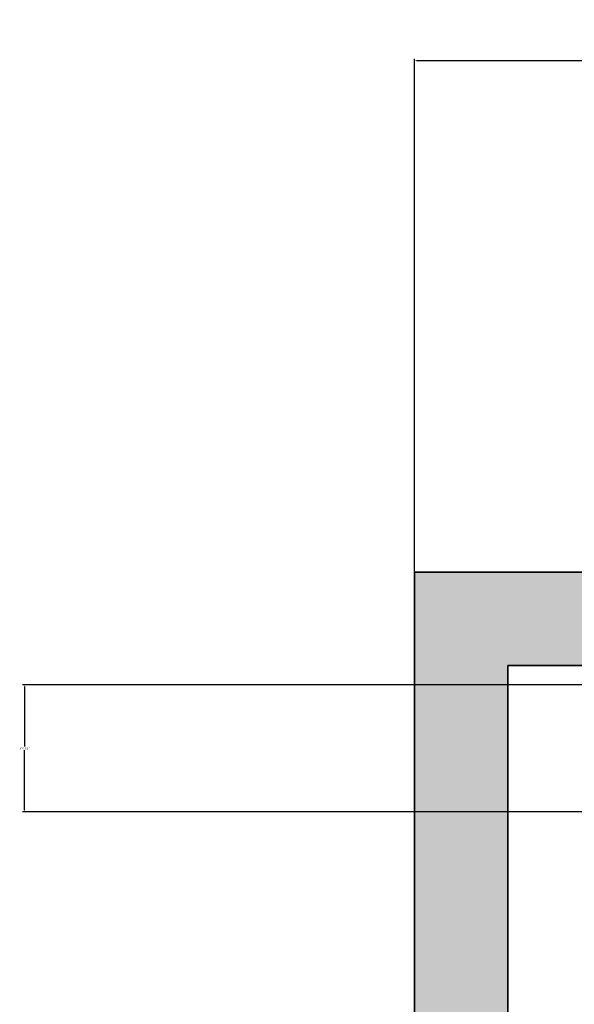
# Model space of a CAD drawing. Units: inches. Extents: x -5 to 482, y -460 to 66.
# Tile 23 of 31: x -5 to 48, y -29 to 66. Entities that reach past the tile are written whole.
import ezdxf

# ---------------------------------------------------------------- set-up
doc = ezdxf.new("R2010")
doc.units = ezdxf.units.IN
doc.header["$MEASUREMENT"] = 0
for name, color, linetype, lineweight in [('A-ANNO-DIMS', 2, 'Continuous', 18), ('A-WALL', 7, 'Continuous', 35), ('A-WALL-PATT', 152, 'Continuous', 13)]:
    doc.layers.add(name, color=color, linetype=linetype, lineweight=lineweight)
doc.styles.get("Standard").update_dxf_attribs({"font": 'arial.ttf'})
doc.dimstyles.get("Standard").update_dxf_attribs({"dimtxt": 0.18, "dimasz": 0.18, "dimexe": 0.18, "dimexo": 0.0625, "dimgap": 0.09, "dimtad": 0, "dimtih": 1, "dimtoh": 1, "dimdec": 0, "dimzin": 0, "dimdsep": 46, "dimlunit": 3, "dimtxsty": 'Standard', "dimcen": 0.09, "dimadec": 0, "dimazin": 0, "dimtfac": 1, "dimtdec": 0, "dimtofl": 0, "dimtmove": 0, "dimatfit": 3, "dimfxl": 1, "dimtolj": 1, "dimtzin": 0, "dimarcsym": 0})

# ---------------------------------------------------------------- blocks, each defined once
blk = doc.blocks.new('*D3')
at = {"layer": 'A-ANNO-DIMS', "color": 0, "lineweight": -2, "transparency": 16777216}
for p, q in [((32.877, 13.214), (32.877, 62.612)), ((33.057, 62.432), (221.233, 62.432)), ((430.197, 62.432), (242.02, 62.432)), ((430.377, 13.214), (430.377, 62.612))]:
    blk.add_line(p, q, dxfattribs=at)
at = {"layer": 'A-ANNO-DIMS', "color": 0, "transparency": 16777216}
for points in [[(33.057, 62.462), (33.057, 62.402), (32.877, 62.432)], [(430.197, 62.462), (430.197, 62.402), (430.377, 62.432)]]:
    blk.add_solid(points, dxfattribs=at)
at = {"layer": 'Defpoints', "color": 0, "transparency": 16777216}
for p in [(430.377, 62.432), (32.877, 13.151), (430.377, 13.151)]:
    blk.add_point(p, dxfattribs=at)
at = {"layer": 'A-ANNO-DIMS', "color": 0, "transparency": 16777216, "insert": (231.627, 62.432), "char_height": 6, "attachment_point": 5}
blk.add_mtext('\\A1;33\'-2"', dxfattribs=at)
blk = doc.blocks.new('*D70')
at = {"layer": 'A-ANNO-DIMS', "color": 0, "lineweight": -2, "transparency": 16777216}
for p, q in [((83.652, 2.288), (-4.903, 2.288)), ((-4.723, 2.108), (-4.723, -3.659)), ((-4.723, -9.792), (-4.723, -4.025)), ((83.652, -9.972), (-4.903, -9.972))]:
    blk.add_line(p, q, dxfattribs=at)
at = {"layer": 'A-ANNO-DIMS', "color": 0, "transparency": 16777216}
for points in [[(-4.753, 2.108), (-4.693, 2.108), (-4.723, 2.288)], [(-4.753, -9.792), (-4.693, -9.792), (-4.723, -9.972)]]:
    blk.add_solid(points, dxfattribs=at)
at = {"layer": 'Defpoints', "color": 0, "transparency": 16777216}
for p in [(83.715, 2.288), (-4.723, -9.972), (83.715, -9.972)]:
    blk.add_point(p, dxfattribs=at)
at = {"layer": 'A-ANNO-DIMS', "color": 0, "transparency": 16777216, "insert": (-4.723, -3.842), "char_height": 0.18, "attachment_point": 5}
blk.add_mtext('\\A1;1\'-0 1/2"', dxfattribs=at)

msp = doc.modelspace()

# ---------------------------------------------------------------- hatches: boundary and pattern name
at = {"layer": 'A-WALL-PATT'}
h = msp.add_hatch(color=256, dxfattribs=at)
h.dxf.hatch_style = 1
h.paths.add_polyline_path([(149.377, -412.849), (144.377, -412.849), (144.377, -283.849), (144.377, -279.349), (133.877, -279.349), (133.877, -283.849), (139.877, -283.849), (139.877, -412.849), (133.51, -412.849), (133.51, -413.916), (102.652, -413.916), (102.652, -421.02), (133.51, -421.02), (133.51, -421.849), (149.377, -421.849)])
h.paths.add_polyline_path([(226.054, -412.849), (218.877, -412.849), (218.877, -350.849), (262.877, -350.849), (262.877, -386.849), (267.377, -386.849), (267.377, -283.849), (270.377, -283.849), (270.377, -279.349), (244.877, -279.349), (244.877, -283.849), (262.877, -283.849), (262.877, -346.349), (218.877, -346.349), (218.877, -283.849), (220.877, -283.849), (220.877, -279.349), (214.377, -279.349), (214.377, -283.849), (214.377, -412.849), (209.377, -412.849), (209.377, -421.849), (226.054, -421.849)])
h.paths.add_polyline_path([(315.815, -412.849), (250.054, -412.849), (250.054, -421.849), (315.815, -421.849)])
h.paths.add_polyline_path([(430.377, -378.349), (421.377, -378.349), (421.377, -412.849), (375.815, -412.849), (375.815, -421.849), (430.377, -421.849)])
h.paths.add_polyline_path([(78.691, -413.916), (47.68, -413.916), (47.68, -412.849), (41.877, -412.849), (41.877, -283.849), (109.877, -283.849), (109.877, -279.349), (41.877, -279.349), (41.877, -241.849), (32.877, -241.849), (32.877, -421.849), (47.68, -421.849), (47.68, -421.02), (78.691, -421.02)])
h.paths.add_polyline_path([(41.877, -144.349), (154.377, -144.349), (154.377, -137.849), (149.877, -137.849), (149.877, -139.849), (41.877, -139.849), (41.877, -97.849), (32.877, -97.849), (32.877, -181.849), (41.877, -181.849)])
h.paths.add_polyline_path([(430.377, -241.849), (421.377, -241.849), (421.377, -279.349), (309.377, -279.349), (309.377, -170.349), (304.877, -170.349), (304.877, -279.349), (294.377, -279.349), (294.377, -283.849), (421.377, -283.849), (421.377, -318.349), (430.377, -318.349)])
h.paths.add_polyline_path([(430.377, -119.849), (421.377, -119.849), (421.377, -139.849), (419.377, -139.849), (419.377, -144.349), (421.377, -144.349), (421.377, -181.849), (430.377, -181.849)])
h.paths.add_polyline_path([(395.377, -139.849), (377.377, -139.849), (377.377, -75.849), (421.377, -75.849), (421.377, -95.849), (430.377, -95.849), (430.377, -45.599), (421.377, -45.599), (421.377, -71.349), (377.377, -71.349), (377.377, -22.849), (372.877, -22.849), (372.877, -139.849), (242.877, -139.849), (242.877, -137.849), (238.377, -137.849), (238.377, -144.349), (304.877, -144.349), (304.877, -146.349), (309.377, -146.349), (309.377, -144.349), (395.377, -144.349)])
h.paths.add_polyline_path([(65.877, 13.151), (32.877, 13.151), (32.877, -37.849), (41.877, -37.849), (41.877, 4.151), (65.877, 4.151)])
h.paths.add_polyline_path([(166.377, 13.151), (125.877, 13.151), (125.877, 4.151), (149.877, 4.151), (149.877, -113.849), (154.377, -113.849), (154.377, 4.151), (166.377, 4.151)])
h.paths.add_polyline_path([(277.877, 13.151), (226.377, 13.151), (226.377, 4.151), (238.377, 4.151), (238.377, -113.849), (242.877, -113.849), (242.877, 4.151), (277.877, 4.151)])
h.paths.add_polyline_path([(430.377, 13.151), (337.877, 13.151), (337.877, 4.151), (372.877, 4.151), (372.877, 1.151), (377.377, 1.151), (377.377, 4.151), (421.377, 4.151), (421.377, -21.599), (430.377, -21.599)])

# ---------------------------------------------------------------- linework, layer by layer
at = {"layer": 'A-WALL'}
for p, q in [((32.877, 13.151), (32.877, -421.849)), ((32.877, 13.151), (430.377, 13.151)), ((41.877, 4.151), (149.877, 4.151)), ((41.877, 4.151), (41.877, -139.849))]:
    msp.add_line(p, q, dxfattribs=at)

# ---------------------------------------------------------------- dimensions: what is measured, and where the dimension line sits
at = {"layer": 'A-ANNO-DIMS'}
dim = msp.add_linear_dim(base=(430.376735986, 62.431571932), p1=(32.876735986, 13.151335974), p2=(430.376735986, 13.151335974), dimstyle='Standard', override={"dimtxt": 6, "dimclrd": 0, "dimclre": 0, "dimclrt": 0}, dxfattribs=at)
dim.commit()
dim.dimension.update_dxf_attribs({"geometry": '*D3', "text_midpoint": (231.626735986, 62.431571932)})
dim = msp.add_linear_dim(base=(-4.723, -9.972), p1=(83.715, 2.288), p2=(83.715, -9.972), angle=90, dimstyle='Standard', override={"dimdec": 1, "dimlfac": 1, "dimrnd": 0, "dimzin": 1, "dimdsep": 46, "dimlunit": 4, "dimfrac": 2}, dxfattribs=at)
dim.commit()
dim.dimension.update_dxf_attribs({"geometry": '*D70', "text_midpoint": (-4.723, -3.842)})

doc.saveas('drawing.dxf')
